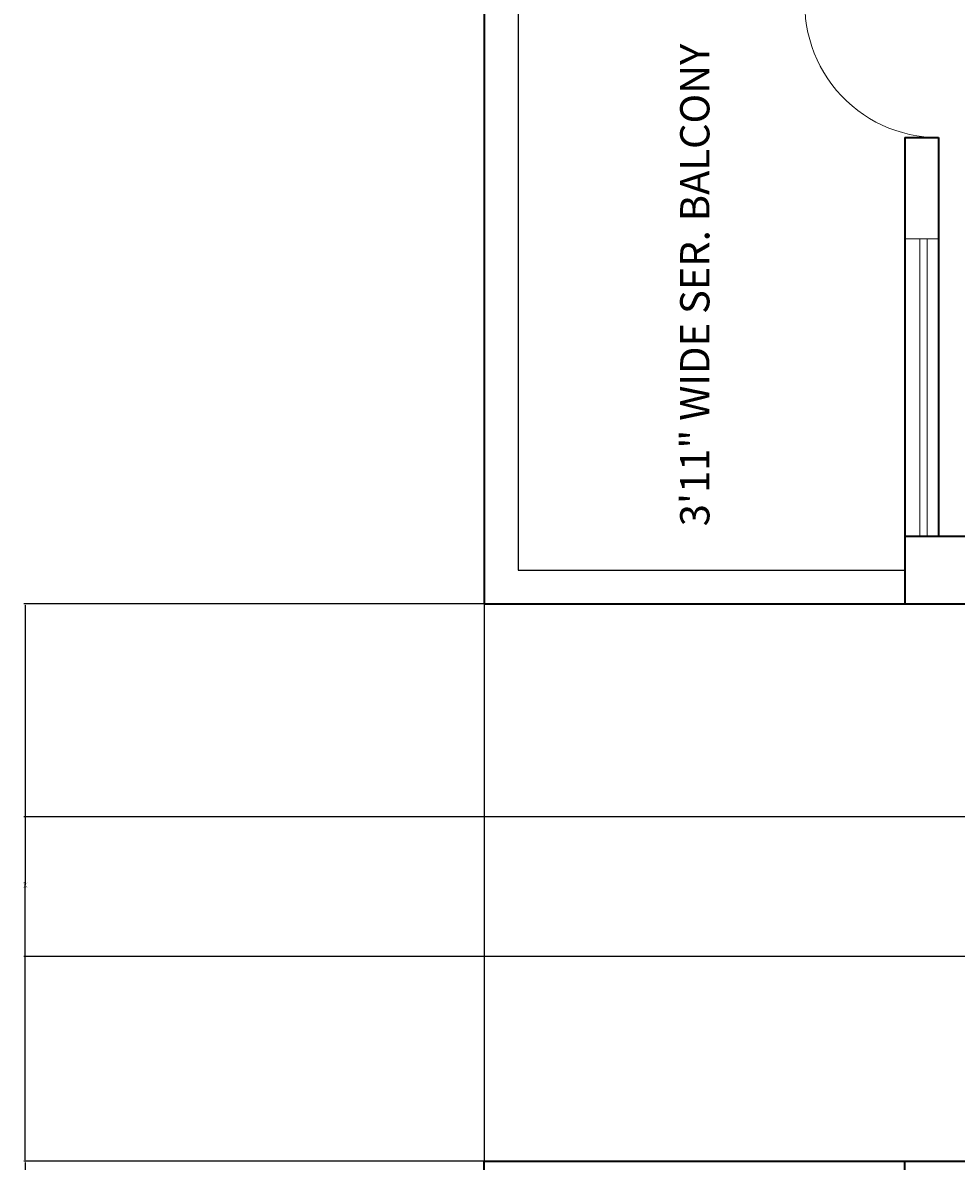
# Model space of a CAD drawing. Units: feet. Extents: x 5816 to 6644, y 25475 to 26788.
# Tile 3 of 23: x 5816 to 5940, y 26094 to 26246. Entities that reach past the tile are written whole.
import ezdxf

# ---------------------------------------------------------------- set-up
doc = ezdxf.new("R2010")
doc.units = ezdxf.units.FT
for name, color, linetype, lineweight in [('A-ANNO-DIMS', 2, 'Continuous', 13), ('A-AREA-IDEN', 7, 'Continuous', 18), ('A-DOOR', 3, 'Continuous', 18), ('A-FLOR-RAIL', 8, 'Continuous', 25), ('A-GLAZ', 4, 'Continuous', 18), ('A-WALL', 7, 'Continuous', 35)]:
    doc.layers.add(name, color=color, linetype=linetype, lineweight=lineweight)
doc.styles.get("Standard").update_dxf_attribs({"font": 'arial.ttf'})
doc.dimstyles.get("Standard").update_dxf_attribs({"dimtxt": 0.18, "dimasz": 0.18, "dimexe": 0.18, "dimexo": 0.0625, "dimgap": 0.09, "dimtad": 0, "dimtih": 1, "dimtoh": 1, "dimdec": 4, "dimzin": 0, "dimdsep": 46, "dimtxsty": 'Standard', "dimcen": 0.09, "dimadec": 0, "dimazin": 0, "dimtfac": 1, "dimtdec": 4, "dimtofl": 0, "dimtmove": 0, "dimatfit": 3, "dimfxl": 1, "dimtolj": 1, "dimtzin": 0, "dimarcsym": 0})

# ---------------------------------------------------------------- blocks, each defined once
blk = doc.blocks.new('DOOR-SERVICE-BALCONY')
blk.add_line((-17.56, 0), (0, 0))
blk.add_arc((0, -2.91), 17.8, 170.5868, 270)
blk = doc.blocks.new('WIN-KITCHEN')
for p, q in [((0, 0), (4.5, 0)), ((2, 0), (2, -39.61)), ((3, 0), (3, -39.61))]:
    blk.add_line(p, q)
blk = doc.blocks.new('*D57')
at = {"layer": 'A-ANNO-DIMS', "color": 0, "lineweight": -2, "transparency": 16777216}
for p, q in [((5877.25, 26168.58), (5815.98, 26168.58)), ((5816.16, 26168.4), (5816.16, 26131.64)), ((5816.16, 26094.52), (5816.16, 26131.28)), ((5877.25, 26094.34), (5815.98, 26094.34))]:
    blk.add_line(p, q, dxfattribs=at)
at = {"layer": 'A-ANNO-DIMS', "color": 0, "transparency": 16777216}
for points in [[(5816.13, 26168.4), (5816.19, 26168.4), (5816.16, 26168.58)], [(5816.13, 26094.52), (5816.19, 26094.52), (5816.16, 26094.34)]]:
    blk.add_solid(points, dxfattribs=at)
at = {"layer": 'Defpoints', "color": 0, "transparency": 16777216}
for p in [(5816.16, 26168.58), (5877.31, 26168.58), (5877.31, 26094.34)]:
    blk.add_point(p, dxfattribs=at)
at = {"layer": 'A-ANNO-DIMS', "color": 0, "transparency": 16777216, "insert": (5816.16, 26131.46), "char_height": 0.18, "attachment_point": 5}
blk.add_mtext('\\A1;74.25', dxfattribs=at)
blk = doc.blocks.new('*D61')
at = {"layer": 'A-ANNO-DIMS', "color": 0, "lineweight": -2, "transparency": 16777216}
for p, q in [((5877.25, 26094.34), (5815.98, 26094.34)), ((5816.16, 26094.16), (5816.16, 25815.52)), ((5816.16, 25536.52), (5816.16, 25815.15)), ((5877.25, 25536.34), (5815.98, 25536.34))]:
    blk.add_line(p, q, dxfattribs=at)
at = {"layer": 'A-ANNO-DIMS', "color": 0, "transparency": 16777216}
for points in [[(5816.13, 26094.16), (5816.19, 26094.16), (5816.16, 26094.34)], [(5816.13, 25536.52), (5816.19, 25536.52), (5816.16, 25536.34)]]:
    blk.add_solid(points, dxfattribs=at)
at = {"layer": 'Defpoints', "color": 0, "transparency": 16777216}
for p in [(5816.16, 26094.34), (5877.31, 26094.34), (5877.31, 25536.34)]:
    blk.add_point(p, dxfattribs=at)
at = {"layer": 'A-ANNO-DIMS', "color": 0, "transparency": 16777216, "insert": (5816.16, 25815.34), "char_height": 0.18, "attachment_point": 5}
blk.add_mtext('\\A1;558', dxfattribs=at)
blk = doc.blocks.new('*D62')
at = {"layer": 'A-ANNO-DIMS', "color": 0, "lineweight": -2, "transparency": 16777216}
for p, q in [((5877.31, 26168.52), (5877.31, 25475.01)), ((5953.98, 26168.52), (5953.98, 25475.01)), ((5877.49, 25475.19), (5915.25, 25475.19)), ((5953.8, 25475.19), (5916.04, 25475.19))]:
    blk.add_line(p, q, dxfattribs=at)
at = {"layer": 'A-ANNO-DIMS', "color": 0, "transparency": 16777216}
for points in [[(5877.49, 25475.22), (5877.49, 25475.16), (5877.31, 25475.19)], [(5953.8, 25475.22), (5953.8, 25475.16), (5953.98, 25475.19)]]:
    blk.add_solid(points, dxfattribs=at)
at = {"layer": 'Defpoints', "color": 0, "transparency": 16777216}
for p in [(5877.31, 26168.58), (5953.98, 26168.58), (5953.98, 25475.19)]:
    blk.add_point(p, dxfattribs=at)
at = {"layer": 'A-ANNO-DIMS', "color": 0, "transparency": 16777216, "insert": (5915.64, 25475.19), "char_height": 0.18, "attachment_point": 5}
blk.add_mtext('\\A1;76.67', dxfattribs=at)
blk = doc.blocks.new('*D71')
at = {"layer": 'A-ANNO-DIMS', "color": 0, "lineweight": -2, "transparency": 16777216}
for p, q in [((6343.61, 26140.22), (5815.98, 26140.22)), ((5816.16, 26140.04), (5816.16, 26131.1)), ((5816.16, 26121.79), (5816.16, 26130.74)), ((6343.61, 26121.61), (5815.98, 26121.61))]:
    blk.add_line(p, q, dxfattribs=at)
at = {"layer": 'A-ANNO-DIMS', "color": 0, "transparency": 16777216}
for points in [[(5816.13, 26140.04), (5816.19, 26140.04), (5816.16, 26140.22)], [(5816.13, 26121.79), (5816.19, 26121.79), (5816.16, 26121.61)]]:
    blk.add_solid(points, dxfattribs=at)
at = {"layer": 'Defpoints', "color": 0, "transparency": 16777216}
for p in [(6343.68, 26140.22), (5816.16, 26121.61), (6343.68, 26121.61)]:
    blk.add_point(p, dxfattribs=at)
at = {"layer": 'A-ANNO-DIMS', "color": 0, "transparency": 16777216, "insert": (5816.16, 26130.92), "char_height": 0.18, "attachment_point": 5}
blk.add_mtext('\\A1;18.61', dxfattribs=at)

msp = doc.modelspace()

# ---------------------------------------------------------------- linework, layer by layer
at = {"layer": 'A-FLOR-RAIL'}
msp.add_lwpolyline([(5881.8119, 26253.5846), (5881.8119, 26173.0846), (5933.3119, 26173.0846)], dxfattribs=at)
at = {"layer": 'A-WALL'}
for p, q in [((5877.3119, 26262.5846), (5877.3119, 26168.5846)), ((5933.3119, 26230.6968), (5937.8119, 26230.6968)), ((5933.3119, 26230.6968), (5933.3119, 26168.5846)), ((5937.8119, 26230.6968), (5937.8119, 26177.5846)), ((5933.3119, 26177.5846), (6047.8119, 26177.5846)), ((5877.3119, 26168.5846), (5953.9781, 26168.5846)), ((5877.3119, 26094.3368), (5933.3119, 26094.3368)), ((5877.3119, 26000.3368), (5877.3119, 26094.3368)), ((5933.3119, 26032.2246), (5933.3119, 26094.3368)), ((5933.3119, 26094.3368), (5953.9781, 26094.3368))]:
    msp.add_line(p, q, dxfattribs=at)

# ---------------------------------------------------------------- block references
at = {"layer": 'A-DOOR'}
msp.add_blockref('DOOR-SERVICE-BALCONY', (5937.8119, 26251.4059), dxfattribs=at)
at = {"layer": 'A-GLAZ'}
msp.add_blockref('WIN-KITCHEN', (5933.3119, 26217.1904), dxfattribs=at)

# ---------------------------------------------------------------- texts
at = {"layer": 'A-AREA-IDEN'}
msp.add_text('3\'11" WIDE SER. BALCONY', height=3.901456, rotation=90, dxfattribs=at).set_placement((5907.3063, 26178.9178))

# ---------------------------------------------------------------- dimensions: what is measured, and where the dimension line sits
at = {"layer": 'A-ANNO-DIMS'}
for base, p1, p2, override, picture, middle in [((5816.1619, 26168.5846), (5877.3119, 26094.3368), (5877.3119, 26168.5846), {"dimdec": 2, "dimlfac": 1, "dimrnd": 0, "dimzin": 0, "dimdsep": 46, "dimlunit": 2}, '*D57', (5816.1619, 26131.4607)), ((5816.1619, 26121.6124), (6343.6763, 26140.2241), (6343.6763, 26121.6124), {"dimdec": 2, "dimlfac": 1, "dimrnd": 0, "dimzin": 0, "dimdsep": 46, "dimlunit": 2}, '*D71', (5816.1619, 26130.9183)), ((5816.1619, 26094.3368), (5877.3119, 25536.3368), (5877.3119, 26094.3368), {"dimdec": 0, "dimlfac": 1, "dimrnd": 0, "dimzin": 0, "dimdsep": 46, "dimlunit": 2}, '*D61', (5816.1619, 25815.3368))]:
    dim = msp.add_linear_dim(base=base, p1=p1, p2=p2, angle=90, dimstyle='Standard', override=override, dxfattribs=at)
    dim.commit()
    dim.dimension.update_dxf_attribs({"geometry": picture, "text_midpoint": middle})
dim = msp.add_linear_dim(base=(5953.9781, 25475.1868), p1=(5877.3119, 26168.5846), p2=(5953.9781, 26168.5846), dimstyle='Standard', override={"dimdec": 2, "dimlfac": 1, "dimrnd": 0, "dimzin": 0, "dimdsep": 46, "dimlunit": 2}, dxfattribs=at)
dim.commit()
dim.dimension.update_dxf_attribs({"geometry": '*D62', "text_midpoint": (5915.645, 25475.1868)})

doc.saveas('drawing.dxf')
